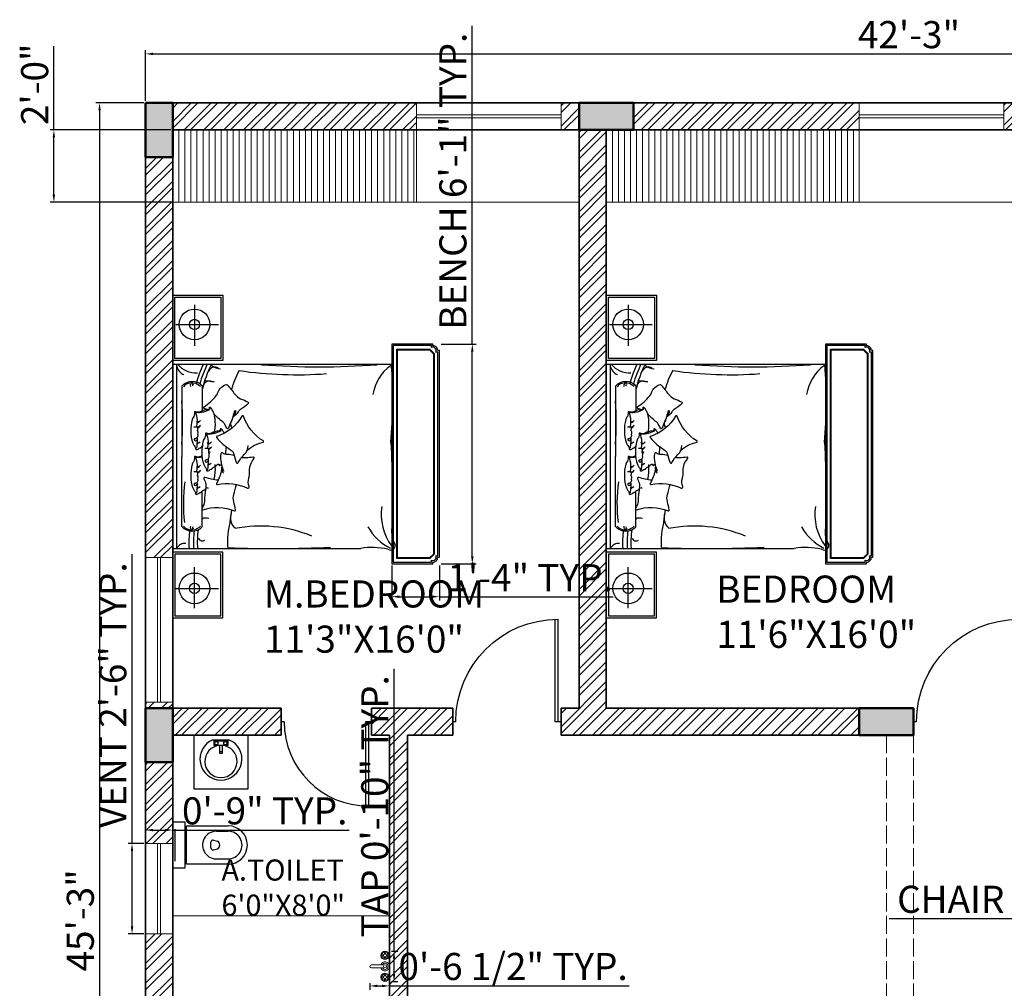
# Model space of a CAD drawing. Units: inches. Extents: x 4153 to 5577, y 785 to 1503.
# Tile 2 of 11: x 4153 to 4480, y 1150 to 1472. Entities that reach past the tile are written whole.
import ezdxf

# ---------------------------------------------------------------- set-up
doc = ezdxf.new("R2010")
doc.units = ezdxf.units.IN
doc.linetypes.add('ACAD_ISO02W100', pattern=[15, 12, -3])
for name, color, linetype, lineweight in [('A-ANNO-DIMS', 2, 'Continuous', 18), ('A-AREA-IDEN', 7, 'Continuous', 25), ('A-COLS', 7, 'Continuous', 50), ('A-DOOR', 3, 'Continuous', 25), ('A-FLOR-CASE', 32, 'Continuous', 18), ('A-FURN', 8, 'Continuous', 18), ('A-GLAZ', 4, 'Continuous', 18), ('A-WALL', 7, 'Continuous', 35), ('A-WALL-OVHD', 7, 'ACAD_ISO02W100', 18), ('Сантехника', 7, 'Continuous', 18)]:
    doc.layers.add(name, color=color, linetype=linetype, lineweight=lineweight)
doc.layers.add('A-FLOR-CASE-PATT', color=32, linetype='Continuous', lineweight=13, true_color=0xcd6928)
doc.layers.add('A-WALL-PATT', color=251, linetype='Continuous', lineweight=13, true_color=0x636466)
for name, color, linetype in [('FUR', 42, 'Continuous'), ('HA-FUR', 8, 'Continuous'), ('HA-P', 8, 'Continuous'), ('SAN', 5, 'Continuous'), ('SANTEH', 7, 'Continuous'), ('wood', 26, 'Continuous')]:
    doc.layers.add(name, color=color, linetype=linetype)
doc.styles.get("Standard").update_dxf_attribs({"font": 'arial.ttf'})
doc.dimstyles.new('ISO-25', dxfattribs={"dimtxt": 9, "dimasz": 2.5, "dimexe": 1.25, "dimexo": 0.625, "dimtad": 1, "dimlunit": 3, "dimtxsty": 'Standard', "dimcen": 2.5, "dimadec": 0, "dimazin": 0, "dimtfac": 1, "dimtmove": 0, "dimatfit": 3, "dimfxl": 1, "dimarcsym": 0})

# ---------------------------------------------------------------- blocks, each defined once
blk = doc.blocks.new('D1')
for p, q in [((1, 0), (1, 34)), ((2, 0), (2, 33.99)), ((0, 0), (2, 0)), ((35, 0), (36, 0))]:
    blk.add_line(p, q)
at = {"ltscale": 0.5}
blk.add_arc((1, 0), 34, 0, 90, dxfattribs=at)
blk = doc.blocks.new('D2')
for p, q in [((1, 0), (1, 28)), ((2, 0), (2, 27.98)), ((0, 0), (2, 0)), ((29, 0), (30, 0))]:
    blk.add_line(p, q)
at = {"ltscale": 0.5}
blk.add_arc((1, 0), 28, 0, 90, dxfattribs=at)
blk = doc.blocks.new('A$C0A42580C')
at = {"layer": 'SAN'}
for p, q in [((0.2873, 0.0301), (0.2873, 0.4484)), ((2.8678, 0.0301), (2.8678, 0.4484)), ((0.0949, 0.2135), (0.4958, 0.2135)), ((3.0601, 0.2135), (2.6592, 0.2135))]:
    blk.add_line(p, q, dxfattribs=at)
for centre, radius in [((0.2873, 0.2135), 0.15), ((2.8678, 0.2135), 0.15), ((0.2873, 0.2135), 0.05), ((2.8678, 0.2135), 0.05)]:
    blk.add_circle(centre, radius, dxfattribs=at)
at = {"layer": 'wood'}
for p, q in [((0.6775, 0.8851), (0.6775, 2.1392)), ((2.4775, 0.8016), (2.4775, 1.838)), ((2.4775, 0), (2.4775, 0.8016)), ((0.888, 0.289), (1.1327, 0.289)), ((1.5, 0.3423), (1.5016, 0.3142)), ((1.6633, 0.3438), (1.6434, 0.3761)), ((2.267, 0.289), (1.9163, 0.289)), ((1.2906, 0.2348), (1.2921, 0.2067)), ((1.4538, 0.2362), (1.434, 0.2685)), ((1.7287, 0.2348), (1.7302, 0.2067)), ((1.8919, 0.2362), (1.8721, 0.2685)), ((0.6775, 0.039), (2.4775, 0.039)), ((0.8909, 0.089), (1.5775, 0.089)), ((2.2642, 0.089), (1.5775, 0.089)), ((0.6775, 0), (2.4775, 0))]:
    blk.add_line(p, q, dxfattribs=at)
blk.add_lwpolyline([(0.6775, 0), (0.6775, 0.8851)], dxfattribs=at)
for points in [[(1.516, 0.7294, -0.128392), (1.4401, 0.8834, 0.70791), (1.427, 0.8863, -0.16964), (1.1848, 0.6919, 0.664036), (1.184, 0.6776, -0.184649), (1.3819, 0.4332, 0.662242), (1.3969, 0.4309, 0.078539), (1.5137, 0.5669, -0.1736), (1.5484, 0.5947, -0.02159), (1.6357, 0.6205, 0.697276), (1.6379, 0.6405, -0.093019), (1.5606, 0.699, 0.216632), (1.4719, 0.7371, -2.511293)], [(1.6795, 0.4818, 0.263265), (1.7191, 0.4839, -0.026108), (1.743, 0.4973, 0.027613), (1.7137, 0.4764, -0.089259), (1.8403, 0.429, 0.662242), (1.8528, 0.4376, -0.162037), (1.8882, 0.732, 0.676499), (1.8733, 0.748, -0.160513), (1.7901, 0.7439, 0.07473), (1.7202, 0.7523, -0.187721), (1.5966, 0.7963, 0.70791), (1.5851, 0.7895, -0.010003), (1.5921, 0.7143, -0.07079), (1.5891, 0.6719, 0.099539)], [(1.1211, 0.3454, 0.032543), (1.1095, 0.3091, -0.658965), (1.0917, 0.3063, 0.074753), (0.9887, 0.4234, 0.100988), (0.953, 0.4429, -0.270711), (0.8753, 0.5273, -0.276825), (0.8775, 0.5337, -0.014937), (0.9701, 0.6081, 0.134834), (1.0135, 0.6643, -0.023706), (1.0474, 0.7372, -0.664036), (1.0616, 0.7394, -0.035987), (1.119, 0.6627, 0.118631), (1.1415, 0.6412, -0.132738), (1.1955, 0.5864)], [(1.1759, 0.5928, 0.013884), (1.1549, 0.6131, 0.174178), (1.1437, 0.6177, 0.104076), (1.1358, 0.6165, 0.389829), (1.1324, 0.6097, 0.296089), (1.1415, 0.6019, -0.036701), (1.1572, 0.5985, -0.040547), (1.3022, 0.543, -0.70791), (1.3021, 0.5296, -0.016811), (1.2631, 0.5085, 0.11866), (1.2414, 0.4904, -0.048791), (1.1649, 0.4055, 0.103757)], [(1.5674, 0.601, 0.057807), (1.5606, 0.5339, -0.173425), (1.5457, 0.49, 0.589988), (1.5538, 0.4706, 0.137312), (1.7236, 0.4985, 0.137312)], [(1.8113, 0.4446, -0.069098), (1.7831, 0.3187, 0.658965), (1.7961, 0.3062, -0.049789), (1.8516, 0.3234, -0.103757), (1.8905, 0.3233, 0.055725), (2.0203, 0.3103, -0.11866), (2.0478, 0.304, 0.016811), (2.0881, 0.2856, 0.70791), (2.0989, 0.2936, -0.16964), (2.1104, 0.604, 0.664036), (2.1001, 0.6139, 0.023706), (2.0214, 0.597, -0.134834), (1.9505, 0.5976, 0.012748), (1.8522, 0.6228)], [(1.3107, 0.4764, 0.145733), (1.3069, 0.4677, 0.488583), (1.3089, 0.4657, -0.012138), (1.3131, 0.4661, -0.125673), (1.3213, 0.4646, -0.750706)], [(1.3153, 0.4751, -0.274893), (1.3379, 0.4529, 0.051436), (1.3468, 0.4293, -0.086628), (1.3532, 0.4078, 0.040196), (1.3593, 0.3772, -0.184744), (1.3556, 0.3344, -2.554464)], [(1.317, 0.4683, -0.060098), (1.3283, 0.4571, -0.16247), (1.3313, 0.4487, 0.120018), (1.3493, 0.3815, -0.060072), (1.3541, 0.3695, -0.13107), (1.3541, 0.3395, -0.024415), (1.3534, 0.3373, 0.070398), (1.3503, 0.3233, 0.528689), (1.3524, 0.3216, -0.069388), (1.3557, 0.3222, -0.158233), (1.4075, 0.3065, 0.085461), (1.4255, 0.2981, 0.147196), (1.6571, 0.3041, 0.10985), (1.6823, 0.3191, -0.179095), (1.7126, 0.3319, -2.318897)], [(1.1013, 0.3688, 0.145733), (1.0975, 0.3601, 0.488583), (1.0995, 0.3581, -0.012138), (1.1036, 0.3585, -0.125673), (1.1119, 0.357, -0.750706)], [(1.1059, 0.3675, -0.274893), (1.1285, 0.3453, 0.051436), (1.1373, 0.3217, -0.086628), (1.1438, 0.3003, 0.040196), (1.1499, 0.2696, -0.184744), (1.1462, 0.2269, -2.554464)], [(1.1076, 0.3607, -0.060098), (1.1189, 0.3495, -0.16247), (1.1219, 0.3411, 0.120018), (1.1399, 0.2739, -0.060072), (1.1447, 0.2619, -0.13107), (1.1447, 0.2319, -0.024415), (1.144, 0.2297, 0.070398), (1.1409, 0.2157, 0.528689), (1.143, 0.2141, -0.069388), (1.1463, 0.2146, -0.158233), (1.1981, 0.1989, 0.085461), (1.2161, 0.1905, 0.147196), (1.4477, 0.1965, 0.10985), (1.4728, 0.2115, -0.179095), (1.5032, 0.2244, -2.318897)], [(1.3509, 0.3219, -0.117141), (1.3688, 0.335, -0.025084), (1.4533, 0.348, 0.033691)], [(1.4359, 0.3803, -0.198519), (1.452, 0.3494, 0.826402), (1.4558, 0.349, 0.095956), (1.4561, 0.3528, 0.242899), (1.4461, 0.3686, -17.523452)], [(1.5447, 0.3525, -0.083557), (1.507, 0.3546, 0.203162), (1.4851, 0.3792, -0.208037), (1.5043, 0.3409, 0.124669), (1.4432, 0.3469, 0.965934)], [(1.5394, 0.3688, 0.145733), (1.5356, 0.3601, 0.488583), (1.5376, 0.3581, -0.012138), (1.5418, 0.3585, -0.125673), (1.55, 0.357, -0.750706)], [(1.5447, 0.3525, -0.008229), (1.5728, 0.3519, 0.033691)], [(1.5728, 0.3519, -0.46905), (1.6152, 0.321, 0.420988), (1.62, 0.3169, 0.857652), (1.6221, 0.3484, 0.548526)], [(1.603, 0.3451, -0.099719), (1.6221, 0.3484, 0.102691)], [(1.6214, 0.3487, -0.010168), (1.6558, 0.3447, 0.033691), (1.6907, 0.3423, -0.220869), (1.7148, 0.3311, -0.288972)], [(1.1415, 0.2143, -0.117141), (1.1594, 0.2274, -0.025084), (1.2439, 0.2405, 0.033691)], [(1.2265, 0.2728, -0.198519), (1.2426, 0.2418, 0.826402), (1.2463, 0.2415, 0.095956), (1.2467, 0.2452, 0.242899), (1.2366, 0.2611, -17.523452)], [(1.3353, 0.2449, -0.083557), (1.2976, 0.247, 0.203162), (1.2757, 0.2717, -0.208037), (1.2948, 0.2333, 0.124669), (1.2338, 0.2393, 0.965934)], [(1.3353, 0.2449, -0.008229), (1.3633, 0.2443, 0.033691)], [(1.3633, 0.2443, -0.46905), (1.4058, 0.2134, 0.420988), (1.4106, 0.2093, 0.857652), (1.4127, 0.2408, 0.548526)], [(1.3936, 0.2375, -0.099719), (1.4127, 0.2408, 0.102691)], [(1.412, 0.2411, -0.010168), (1.4464, 0.2371, 0.033691), (1.4812, 0.2348, -0.220869), (1.5054, 0.2235, -0.288972)], [(1.5721, 0.286, 0.022869), (1.578, 0.2739, -0.060072), (1.5828, 0.2619, -0.13107), (1.5828, 0.2319, -0.024415), (1.5821, 0.2297, 0.070398), (1.579, 0.2157, 0.528689), (1.5811, 0.2141, -0.069388), (1.5844, 0.2146, -0.158233), (1.6362, 0.1989, 0.085461), (1.6542, 0.1905, 0.147196), (1.8858, 0.1965, 0.10985), (1.911, 0.2115, -0.179095), (1.9413, 0.2244, -2.318897)], [(1.5796, 0.2143, -0.117141), (1.5975, 0.2274, -0.025084), (1.682, 0.2405, 0.033691)], [(1.5838, 0.2873, 0.023398), (1.588, 0.2696, -0.184744), (1.5843, 0.2269, -2.554464)], [(1.6646, 0.2728, -0.198519), (1.6807, 0.2418, 0.826402), (1.6845, 0.2415, 0.095956), (1.6848, 0.2452, 0.242899), (1.6748, 0.2611, -17.523452)], [(1.7734, 0.2449, -0.083557), (1.7357, 0.247, 0.203162), (1.7138, 0.2717, -0.208037), (1.733, 0.2333, 0.124669), (1.6719, 0.2393, 0.965934)], [(1.7734, 0.2449, -0.008229), (1.8015, 0.2443, 0.033691)], [(1.8015, 0.2443, -0.46905), (1.8439, 0.2134, 0.420988), (1.8487, 0.2093, 0.857652), (1.8508, 0.2408, 0.548526)], [(1.8317, 0.2375, -0.099719), (1.8508, 0.2408, 0.102691)], [(1.8501, 0.2411, -0.010168), (1.8845, 0.2371, 0.033691), (1.9193, 0.2348, -0.220869), (1.9435, 0.2235, -0.288972)]]:
    blk.add_lwpolyline(points, format="xyb", dxfattribs=at)
for points in [[(0.64, 0), (0, 0), (0, 0.49), (0.64, 0.49)], [(2.515, 0), (3.155, 0), (3.155, 0.49), (2.515, 0.49)], [(0.62, 0.02), (0.02, 0.02), (0.02, 0.47), (0.62, 0.47)], [(2.535, 0.02), (3.135, 0.02), (3.135, 0.47), (2.535, 0.47)]]:
    blk.add_lwpolyline(points, close=True, dxfattribs=at)
for centre, radius, start, end in [((1.0344, -2.14), 4.292, 84.56078, 94.7164), ((1.0494, 2.4026), 0.4515, 217.47941, 260.35986), ((2.0208, -11.0786), 13.2288, 88.75549, 92.51133), ((2.1491, 2.5471), 0.5083, 260.65485, 306.44155), ((2.3125, 2.3833), 0.2443, 254.1515, 300.95574), ((2.0168, 2.3573), 0.5127, 299.08175, 333.44367), ((2.4501, 2.1309), 0.0445, 324.18954, 118.92203), ((3.1371, 1.9502), 0.669, 166.6404, 189.65708), ((-7.0839, 1.4328), 7.7858, 355.84817, 4.15183), ((-7.2439, 0.9937), 9.7233, 357.34474, 3.23068), ((-3.167, 1.2143), 3.9465, 351.77286, 4.18386), ((3.5803, 0.8622), 1.3213, 157.81295, 191.15154), ((1.1611, 1.4181), 0.8768, 241.21362, 254.41879), ((1.7861, -2.1601), 2.7557, 80.89877, 83.46656), ((2.181, 0.6859), 0.1221, 247.37754, 321.13165), ((1.2583, 0.6364), 0.0695, 238.58923, 301.92671), ((1.3546, 0.4469), 0.0529, 114.21284, 146.15395), ((2.6126, -2.3504), 3.1201, 113.83178, 114.21284), ((1.4714, 0.0722), 0.4528, 80.62397, 88.74059), ((1.4035, -0.3388), 0.8693, 79.71489, 80.62397), ((1.6301, 0.4539), 0.0342, 31.14095, 54.95422), ((2.4192, 1.3819), 0.8461, 255.77539, 273.25587), ((0.5904, 0.4689), 0.13, 317.38218, 359.70393), ((0.7723, 0.4131), 0.0674, 147.68233, 245.79865), ((0.0312, 0.4583), 0.8174, 350.42368, 356.2506), ((1.1452, 0.3394), 0.0529, 114.21284, 146.15395), ((2.4032, -2.458), 3.1201, 113.55686, 114.21284), ((1.2046, 0.2912), 0.121, 99.42032, 113.55686), ((1.2774, -0.1478), 0.5659, 95.90379, 99.42032), ((1.2626, -0.005), 0.4223, 88.74059, 95.90379), ((1.2619, -0.0354), 0.4528, 80.62397, 88.74059), ((1.1941, -0.4464), 0.8693, 79.45871, 80.62397), ((1.6709, 0.4489), 0.0156, 131.9623, 212.08127), ((1.6729, 0.4422), 0.0178, 140.41793, 157.63267), ((1.7007, -0.005), 0.4223, 88.74059, 95.90379), ((1.7235, 0.4818), 0.0777, 212.08127, 227.364), ((1.6635, 0.4499), 0.00568, 95.52245, 140.41793), ((1.5664, 0.4154), 0.1086, 24.20989, 31.14095), ((1.6627, 0.4587), 0.00309, 275.52245, 24.20989), ((1.6391, 0.3902), 0.0469, 17.32618, 47.364), ((1.7106, 0.4125), 0.028, 197.32618, 226.17302), ((1.6431, 0.3422), 0.0695, 26.61764, 46.17302), ((1.7001, -0.0354), 0.4528, 80.62397, 88.74059), ((1.6322, -0.4464), 0.8693, 78.43923, 80.62397), ((1.1611, 1.3191), 1.0568, 242.76671, 257.10398), ((1.1611, 1.3191), 1.0937, 243.75553, 254.4906), ((1.1611, 1.2816), 1.0937, 243.75553, 254.38927), ((0.9021, 0.3562), 0.0605, 155.8342, 254.41058), ((0.9846, 0.1903), 0.1381, 134.39284, 227.23745), ((1.4207, 0.3463), 0.0342, 31.14095, 54.95422), ((1.4614, 0.3413), 0.0156, 131.9623, 212.08127), ((1.4635, 0.3347), 0.0178, 140.41793, 157.63267), ((1.4541, 0.3424), 0.00568, 95.52245, 140.41793), ((1.357, 0.3078), 0.1086, 24.20989, 31.14095), ((1.4533, 0.3511), 0.00309, 275.52245, 24.20989), ((1.5012, 0.305), 0.028, 197.32618, 226.17302), ((1.8202, 0.431), 0.1287, 206.61764, 215.96192), ((1.715, 0.3349), 0.00379, 207.1817, 328.02977), ((1.6975, 0.3419), 0.023, 350.76434, 35.96192), ((1.7058, 0.3406), 0.0145, 328.02977, 350.76434), ((1.9016, 0.3347), 0.0178, 140.41793, 157.63267), ((1.9522, 0.3743), 0.0777, 212.08127, 227.364), ((1.8922, 0.3424), 0.00568, 95.52245, 140.41793), ((1.8678, 0.2827), 0.0469, 17.32618, 47.364), ((1.9393, 0.305), 0.028, 197.32618, 226.17302), ((2.2511, 0.3256), 0.071, 155.86842, 211.04513), ((2.1704, 0.1903), 0.1381, 312.76255, 45.60716), ((2.3616, 0.2915), 0.0419, 290.78583, 35.36309), ((0.5293, 0.2241), 0.2307, 309.63048, 4.27465), ((0.8396, 0.185), 0.0112, 314.89662, 45.10338), ((0.8413, 0.1846), 0.0128, 299.47062, 57.44416), ((0.8802, 0.1371), 0.0592, 81.47786, 123.11925), ((0.8698, 0.1793), 0.0229, 77.14902, 159.1786), ((0.9986, 0.1735), 0.1427, 136.58239, 164.9725), ((1.4337, 0.2347), 0.0695, 26.61764, 46.17302), ((1.6108, 0.3235), 0.1287, 206.61764, 215.96192), ((1.5055, 0.2273), 0.00379, 207.1817, 328.02977), ((1.4881, 0.2344), 0.023, 350.76434, 35.96192), ((1.4964, 0.233), 0.0145, 328.02977, 350.76434), ((1.8718, 0.2347), 0.0695, 26.61764, 46.17302), ((2.0489, 0.3235), 0.1287, 206.61764, 215.96192), ((1.9436, 0.2273), 0.00379, 207.1817, 328.02977), ((1.9262, 0.2344), 0.023, 350.76434, 35.96192), ((1.9345, 0.233), 0.0145, 328.02977, 350.76434), ((2.1565, 0.1735), 0.1427, 15.0275, 43.41761), ((2.2749, 0.1371), 0.0592, 56.88075, 98.52214), ((2.2853, 0.1793), 0.0229, 20.8214, 102.85098), ((2.4192, 1.2667), 1.0261, 263.09035, 273.25587), ((2.3138, 0.1846), 0.0128, 122.55584, 240.52938), ((2.3154, 0.185), 0.0112, 134.89662, 225.10338), ((2.4192, 1.2667), 1.0629, 263.94374, 273.25587), ((0.6729, 0.151), 0.1135, 279.23824, 338.73819), ((0.8844, 0.2286), 0.0569, 229.70587, 281.11527), ((0.9466, 0.1765), 0.0862, 185.53723, 234.68694), ((1.2481, -2.5919), 2.6893, 85.4722, 94.5278), ((2.0447, 1.7022), 1.5979, 262.13639, 276.48786), ((2.2085, 0.1765), 0.0862, 305.31306, 354.46277), ((2.2706, 0.2286), 0.0569, 258.88473, 310.29413), ((2.4192, 1.2218), 1.0629, 263.23622, 273.25587), ((2.508, 0.1152), 0.0792, 169.94668, 248.24015)]:
    blk.add_arc(centre, radius, start, end, dxfattribs=at)
blk = doc.blocks.new('A$C623F1DA0')
at = {"layer": 'FUR'}
blk.add_lwpolyline([(0.628, 2.912, 0.414214), (0.562, 2.978), (0.562, 3), (0, 3), (0, 0), (0.562, 0), (0.562, 0.022, 0.414214), (0.628, 0.088), (0.65, 0.088), (0.65, 2.912)], format="xyb", close=True, dxfattribs=at)
at = {"layer": 'HA-FUR'}
blk.add_lwpolyline([(0.603, 2.892, 0.710288), (0.542, 2.953), (0.542, 2.98), (0.02, 2.98), (0.02, 0.02), (0.542, 0.02), (0.542, 0.047, 0.710288), (0.603, 0.108), (0.63, 0.108), (0.63, 2.892)], format="xyb", close=True, dxfattribs=at)
at = {"layer": 'HA-P'}
for points in [[(0.07, 2.93), (0.521, 2.93), (0.58, 2.871), (0.58, 0.129), (0.521, 0.07), (0.07, 0.07)], [(0.08, 2.92), (0.517, 2.92), (0.57, 2.867), (0.57, 0.133), (0.517, 0.08), (0.08, 0.08)]]:
    blk.add_lwpolyline(points, close=True, dxfattribs=at)
blk = doc.blocks.new('Faucet - Bathroom top')
for p, q in [((-4.107, 0.125), (-4.375, 0.125)), ((-3.75, 0.4788), (-3.75, 0.75)), ((-3.5, 0.482), (-3.5, 0.75)), ((-3.1461, 0.125), (-2.875, 0.125)), ((3.143, 0.125), (2.875, 0.125)), ((3.5, 0.4788), (3.5, 0.75)), ((3.75, 0.482), (3.75, 0.75)), ((4.1039, 0.125), (4.375, 0.125)), ((-4.1039, -0.125), (-4.375, -0.125)), ((-3.75, -0.4821), (-3.75, -0.75)), ((-3.5, -0.4789), (-3.5, -0.75)), ((-3.143, -0.125), (-2.875, -0.125)), ((-0.5, -0.8639), (-0.5, -4.5)), ((0.5, -4.5), (0.5, -0.8631)), ((3.1461, -0.125), (2.875, -0.125)), ((3.5, -0.4821), (3.5, -0.75)), ((3.75, -0.4789), (3.75, -0.75)), ((4.107, -0.125), (4.375, -0.125))]:
    blk.add_line(p, q)
for centre, radius in [((-3.625, 0), 1.375), ((-4.625, 0), 0.2795), ((-3.625, 0), 0.5), ((-3.625, 1), 0.2795), ((-2.625, 0), 0.2795), ((0, 0), 0.5), ((3.625, 0), 1.375), ((2.625, 0), 0.2795), ((3.625, 0), 0.5), ((3.625, 1), 0.2795), ((4.625, 0), 0.2795), ((-3.625, -1), 0.2795), ((3.625, -1), 0.2795)]:
    blk.add_circle(centre, radius)
for centre, radius, start, end in [((-3.625, 0), 1, 105.2407, 164.2093), ((-3.625, 0), 1, 16.44125, 74.07887), ((0, 0), 1.5, 289.6514, 250.3603), ((0, 0), 1, 300.3431, 239.7554), ((3.625, 0), 1, 106.12, 164.0884), ((3.625, 0), 1, 16.23422, 73.90469), ((-3.625, 0), 1, 196.2342, 253.9047), ((-3.625, 0), 1, 286.12, 344.0884), ((3.625, 0), 1, 196.4413, 254.0789), ((3.625, 0), 1, 285.2407, 344.2093), ((0, -4.5), 0.5, 180, 0)]:
    blk.add_arc(centre, radius, start, end)
blk = doc.blocks.new('y3')
at = {"layer": 'SANTEH', "ltscale": 5}
for p, q in [((37.5, 130.7), (37.5, 520.7)), ((87.5, 410.7), (87.5, 520.7)), ((346.6, 426.1), (347.5, 520.7)), ((397.5, 520.7), (397.5, 130.7)), ((171.9, 384.5), (181.1, 421.3)), ((263.1, 384.5), (253.9, 421.3)), ((244.3, 357.8), (190.7, 357.8)), ((397.5, 130.7), (37.5, 130.7)), ((67.5, 20.7), (367.5, 20.7))]:
    blk.add_line(p, q, dxfattribs=at)
blk.add_lwpolyline([(0, 115), (435, 115), (435, 0), (0, 0), (0, 115)], dxfattribs=at)
for centre, radius, start, end in [((217.5, 520.7), 180, 0, 180), ((217.5, 520.7), 130, 359.15795, 180), ((217.5, 410.7), 130, 180, 5.98548), ((190.7, 377.8), 20, 160.50385, 270), ((217.5, 399.9), 42.2, 30.52342, 149.47658), ((244.3, 377.8), 20, 270, 19.49615)]:
    blk.add_arc(centre, radius, start, end, dxfattribs=at)
blk = doc.blocks.new('r11')
at = {"layer": 'SANTEH', "ltscale": 5}
for p, q in [((0, 0), (600, 0)), ((0, -600), (0, 0)), ((600, 0), (600, -600)), ((210, -50), (390, -50)), ((210, -50), (210, -50)), ((224, -63), (376, -63)), ((224, -113), (224, -63)), ((233, -79), (249, -69)), ((233, -98), (233, -79)), ((249, -107), (233, -98)), ((249, -69), (266, -79)), ((266, -98), (249, -107)), ((266, -79), (266, -98)), ((334, -79), (351, -69)), ((334, -98), (334, -79)), ((351, -107), (334, -98)), ((351, -69), (367, -79)), ((367, -98), (351, -107)), ((367, -79), (367, -98)), ((376, -63), (376, -113)), ((376, -113), (224, -113)), ((288, -202), (288, -113)), ((312, -184), (288, -184)), ((312, -202), (288, -202)), ((312, -113), (312, -202)), ((600, -600), (0, -600))]:
    blk.add_line(p, q, dxfattribs=at)
for centre, radius, start, end in [((300, -266), 234, 112.5, 67.5), ((300, -293), 180, 93.8183, 86.1817)]:
    blk.add_arc(centre, radius, start, end, dxfattribs=at)
blk = doc.blocks.new('*D21')
at = {"layer": 'A-ANNO-DIMS', "color": 0, "lineweight": -2, "transparency": 16777216}
for p, q in [((4194.93, 1445.11), (4194.93, 1461.99)), ((4701.93, 1445.11), (4701.93, 1461.99)), ((4197.43, 1460.74), (4699.43, 1460.74))]:
    blk.add_line(p, q, dxfattribs=at)
at = {"layer": 'A-ANNO-DIMS', "color": 0, "transparency": 16777216}
for points in [[(4197.43, 1461.16), (4197.43, 1460.33), (4194.93, 1460.74)], [(4699.43, 1461.16), (4699.43, 1460.33), (4701.93, 1460.74)]]:
    blk.add_solid(points, dxfattribs=at)
at = {"layer": 'Defpoints', "color": 0, "transparency": 16777216}
for p in [(4701.93, 1460.74), (4194.93, 1444.49), (4701.93, 1444.49)]:
    blk.add_point(p, dxfattribs=at)
at = {"layer": 'A-ANNO-DIMS', "color": 0, "transparency": 16777216, "insert": (4448.43, 1465.97), "char_height": 9, "attachment_point": 5}
blk.add_mtext('42\'-3"', dxfattribs=at)
blk = doc.blocks.new('*D22')
at = {"layer": 'A-ANNO-DIMS', "color": 0, "lineweight": -2, "transparency": 16777216}
for p, q in [((4194.3, 1444.49), (4178.39, 1444.49)), ((4179.64, 1441.99), (4179.64, 903.99)), ((4194.3, 901.49), (4178.39, 901.49))]:
    blk.add_line(p, q, dxfattribs=at)
at = {"layer": 'A-ANNO-DIMS', "color": 0, "transparency": 16777216}
for points in [[(4179.23, 1441.99), (4180.06, 1441.99), (4179.64, 1444.49)], [(4179.23, 903.99), (4180.06, 903.99), (4179.64, 901.49)]]:
    blk.add_solid(points, dxfattribs=at)
at = {"layer": 'Defpoints', "color": 0, "transparency": 16777216}
for p in [(4194.93, 1444.49), (4179.64, 901.49), (4194.93, 901.49)]:
    blk.add_point(p, dxfattribs=at)
at = {"layer": 'A-ANNO-DIMS', "color": 0, "transparency": 16777216, "insert": (4174.42, 1172.99), "char_height": 9, "attachment_point": 5, "rotation": 90}
blk.add_mtext('45\'-3"', dxfattribs=at)
blk = doc.blocks.new('WINDOW-48IN')
for p, q in [((0, 9), (0, 0)), ((48, 9), (48, 0)), ((0, 5), (48, 5)), ((0, 4), (48, 4))]:
    blk.add_line(p, q)
blk = doc.blocks.new('VENT-WINDOW-30IN')
for p, q in [((9, 30), (0, 30)), ((4, 0), (4, 30)), ((5, 0), (5, 30)), ((9, 0), (0, 0))]:
    blk.add_line(p, q)
blk = doc.blocks.new('COL-9X18IN')
at = {"transparency": 33554687}
h = blk.add_hatch(color=256, dxfattribs=at)
h.dxf.hatch_style = 1
h.paths.add_polyline_path([(9, 18), (0, 18), (0, 0), (9, 0)])
blk.add_lwpolyline([(0, 18), (9, 18), (9, 0), (0, 0)], close=True)
blk = doc.blocks.new('*D110')
at = {"layer": 'A-ANNO-DIMS', "color": 0, "lineweight": -2, "transparency": 16777216}
for p, q in [((4190.43, 1198.49), (4190.43, 1294.59)), ((4194.3, 1198.49), (4189.18, 1198.49)), ((4190.43, 1170.99), (4190.43, 1195.99)), ((4194.3, 1168.49), (4189.18, 1168.49))]:
    blk.add_line(p, q, dxfattribs=at)
at = {"layer": 'A-ANNO-DIMS', "color": 0, "transparency": 16777216}
for points in [[(4190.01, 1195.99), (4190.84, 1195.99), (4190.43, 1198.49)], [(4190.01, 1170.99), (4190.84, 1170.99), (4190.43, 1168.49)]]:
    blk.add_solid(points, dxfattribs=at)
at = {"layer": 'Defpoints', "color": 0, "transparency": 16777216}
for p in [(4190.43, 1198.49), (4194.93, 1198.49), (4194.93, 1168.49)]:
    blk.add_point(p, dxfattribs=at)
at = {"layer": 'A-ANNO-DIMS', "color": 0, "transparency": 16777216, "insert": (4185.21, 1247.79), "char_height": 9, "attachment_point": 5, "rotation": 90}
blk.add_mtext('VENT 2\'-6" TYP.', dxfattribs=at)
blk = doc.blocks.new('*D111')
at = {"layer": 'A-ANNO-DIMS', "color": 0, "lineweight": -2, "transparency": 16777216}
for p, q in [((4194.93, 1199.11), (4194.93, 1204.24)), ((4203.93, 1199.11), (4203.93, 1204.24)), ((4197.43, 1202.99), (4201.43, 1202.99)), ((4203.93, 1202.99), (4262.54, 1202.99))]:
    blk.add_line(p, q, dxfattribs=at)
at = {"layer": 'A-ANNO-DIMS', "color": 0, "transparency": 16777216}
for points in [[(4197.43, 1203.41), (4197.43, 1202.57), (4194.93, 1202.99)], [(4201.43, 1203.41), (4201.43, 1202.57), (4203.93, 1202.99)]]:
    blk.add_solid(points, dxfattribs=at)
at = {"layer": 'Defpoints', "color": 0, "transparency": 16777216}
for p in [(4203.93, 1202.99), (4194.93, 1198.49), (4203.93, 1198.49)]:
    blk.add_point(p, dxfattribs=at)
at = {"layer": 'A-ANNO-DIMS', "color": 0, "transparency": 16777216, "insert": (4234.48, 1208.21), "char_height": 9, "attachment_point": 5}
blk.add_mtext('0\'-9" TYP.', dxfattribs=at)
blk = doc.blocks.new('*D114')
at = {"layer": 'A-ANNO-DIMS', "color": 0, "lineweight": -2, "transparency": 16777216}
for p, q in [((4303.43, 1364.36), (4303.43, 1470.08)), ((4293.11, 1364.36), (4304.68, 1364.36)), ((4303.43, 1293.93), (4303.43, 1361.86)), ((4293.11, 1291.43), (4304.68, 1291.43))]:
    blk.add_line(p, q, dxfattribs=at)
at = {"layer": 'A-ANNO-DIMS', "color": 0, "transparency": 16777216}
for points in [[(4303.01, 1361.86), (4303.84, 1361.86), (4303.43, 1364.36)], [(4303.01, 1293.93), (4303.84, 1293.93), (4303.43, 1291.43)]]:
    blk.add_solid(points, dxfattribs=at)
at = {"layer": 'Defpoints', "color": 0, "transparency": 16777216}
for p in [(4292.49, 1364.36), (4303.43, 1364.36), (4292.49, 1291.43)]:
    blk.add_point(p, dxfattribs=at)
at = {"layer": 'A-ANNO-DIMS', "color": 0, "transparency": 16777216, "insert": (4298.15, 1418.47), "char_height": 9, "attachment_point": 5, "rotation": 90}
blk.add_mtext('BENCH 6\'-1" TYP.', dxfattribs=at)
blk = doc.blocks.new('*D115')
at = {"layer": 'A-ANNO-DIMS', "color": 0, "lineweight": -2, "transparency": 16777216}
for p, q in [((4276.69, 1290.81), (4276.69, 1279.24)), ((4292.49, 1290.81), (4292.49, 1279.24)), ((4279.19, 1280.49), (4289.99, 1280.49)), ((4292.49, 1280.49), (4350.25, 1280.49))]:
    blk.add_line(p, q, dxfattribs=at)
at = {"layer": 'A-ANNO-DIMS', "color": 0, "transparency": 16777216}
for points in [[(4279.19, 1280.91), (4279.19, 1280.08), (4276.69, 1280.49)], [(4289.99, 1280.91), (4289.99, 1280.08), (4292.49, 1280.49)]]:
    blk.add_solid(points, dxfattribs=at)
at = {"layer": 'Defpoints', "color": 0, "transparency": 16777216}
for p in [(4276.69, 1291.43), (4292.49, 1291.43), (4292.49, 1280.49)]:
    blk.add_point(p, dxfattribs=at)
at = {"layer": 'A-ANNO-DIMS', "color": 0, "transparency": 16777216, "insert": (4322.62, 1285.64), "char_height": 9, "attachment_point": 5}
blk.add_mtext('1\'-4" TYP.', dxfattribs=at)
blk = doc.blocks.new('*D116')
at = {"layer": 'A-ANNO-DIMS', "color": 0, "lineweight": -2, "transparency": 16777216}
for p, q in [((4277.43, 1162.74), (4277.43, 1256.51)), ((4276.55, 1162.74), (4278.68, 1162.74)), ((4277.43, 1155.24), (4277.43, 1160.24)), ((4276.55, 1152.74), (4278.68, 1152.74))]:
    blk.add_line(p, q, dxfattribs=at)
at = {"layer": 'A-ANNO-DIMS', "color": 0, "transparency": 16777216}
for points in [[(4277.01, 1160.24), (4277.84, 1160.24), (4277.43, 1162.74)], [(4277.01, 1155.24), (4277.84, 1155.24), (4277.43, 1152.74)]]:
    blk.add_solid(points, dxfattribs=at)
at = {"layer": 'Defpoints', "color": 0, "transparency": 16777216}
for p in [(4275.93, 1162.74), (4277.43, 1162.74), (4275.93, 1152.74)]:
    blk.add_point(p, dxfattribs=at)
at = {"layer": 'A-ANNO-DIMS', "color": 0, "transparency": 16777216, "insert": (4272.21, 1210.88), "char_height": 9, "attachment_point": 5, "rotation": 90}
blk.add_mtext('TAP 0\'-10" TYP.', dxfattribs=at)
blk = doc.blocks.new('*D117')
at = {"layer": 'A-ANNO-DIMS', "color": 0, "lineweight": -2, "transparency": 16777216}
for p, q in [((4269.43, 1152.11), (4269.43, 1149.99)), ((4271.93, 1151.24), (4273.43, 1151.24)), ((4275.93, 1152.11), (4275.93, 1149.99)), ((4275.93, 1151.24), (4355.51, 1151.24))]:
    blk.add_line(p, q, dxfattribs=at)
at = {"layer": 'A-ANNO-DIMS', "color": 0, "transparency": 16777216}
for points in [[(4271.93, 1151.66), (4271.93, 1150.82), (4269.43, 1151.24)], [(4273.43, 1151.66), (4273.43, 1150.82), (4275.93, 1151.24)]]:
    blk.add_solid(points, dxfattribs=at)
at = {"layer": 'Defpoints', "color": 0, "transparency": 16777216}
for p in [(4269.43, 1152.74), (4275.93, 1152.74), (4275.93, 1151.24)]:
    blk.add_point(p, dxfattribs=at)
at = {"layer": 'A-ANNO-DIMS', "color": 0, "transparency": 16777216, "insert": (4316.97, 1156.52), "char_height": 9, "attachment_point": 5}
blk.add_mtext('0\'-6 1/2" TYP.', dxfattribs=at)
blk = doc.blocks.new('*D128')
at = {"layer": 'A-ANNO-DIMS', "color": 0, "lineweight": -2, "transparency": 16777216}
for p, q in [((4542.96, 1178.31), (4542.96, 1172.3)), ((4578.86, 1178.31), (4578.86, 1172.3)), ((4542.96, 1173.55), (4441.84, 1173.55)), ((4576.36, 1173.55), (4545.46, 1173.55))]:
    blk.add_line(p, q, dxfattribs=at)
at = {"layer": 'A-ANNO-DIMS', "color": 0, "transparency": 16777216}
for points in [[(4545.46, 1173.96), (4545.46, 1173.13), (4542.96, 1173.55)], [(4576.36, 1173.96), (4576.36, 1173.13), (4578.86, 1173.55)]]:
    blk.add_solid(points, dxfattribs=at)
at = {"layer": 'Defpoints', "color": 0, "transparency": 16777216}
for p in [(4542.96, 1178.93), (4578.86, 1178.93), (4542.96, 1173.55)]:
    blk.add_point(p, dxfattribs=at)
at = {"layer": 'A-ANNO-DIMS', "color": 0, "transparency": 16777216, "insert": (4491.15, 1178.83), "char_height": 9, "attachment_point": 5}
blk.add_mtext('CHAIR 3\'-0" TYP.', dxfattribs=at)
blk = doc.blocks.new('*D161')
at = {"layer": 'A-ANNO-DIMS', "color": 0, "lineweight": -2, "transparency": 16777216}
for p, q in [((4164.48, 1435.49), (4164.48, 1463.32)), ((4203.3, 1435.49), (4163.23, 1435.49)), ((4164.48, 1413.99), (4164.48, 1432.99)), ((4203.3, 1411.49), (4163.23, 1411.49))]:
    blk.add_line(p, q, dxfattribs=at)
at = {"layer": 'A-ANNO-DIMS', "color": 0, "transparency": 16777216}
for points in [[(4164.06, 1432.99), (4164.89, 1432.99), (4164.48, 1435.49)], [(4164.06, 1413.99), (4164.89, 1413.99), (4164.48, 1411.49)]]:
    blk.add_solid(points, dxfattribs=at)
at = {"layer": 'Defpoints', "color": 0, "transparency": 16777216}
for p in [(4164.48, 1435.49), (4203.93, 1435.49), (4203.93, 1411.49)]:
    blk.add_point(p, dxfattribs=at)
at = {"layer": 'A-ANNO-DIMS', "color": 0, "transparency": 16777216, "insert": (4159.26, 1450.65), "char_height": 9, "attachment_point": 5, "rotation": 90}
blk.add_mtext('2\'-0"', dxfattribs=at)

msp = doc.modelspace()

# ---------------------------------------------------------------- hatches: boundary and pattern name
at = {"layer": 'A-FLOR-CASE-PATT'}
h = msp.add_hatch(dxfattribs=at)
h.set_pattern_fill('ANSI31', color=256, scale=0.629921, angle=45, style=0)
h.paths.add_polyline_path([(4203.927, 1411.488), (4284.927, 1411.488), (4284.927, 1435.488), (4203.927, 1435.488)])
h = msp.add_hatch(dxfattribs=at)
h.set_pattern_fill('ANSI31', color=256, scale=0.629921, angle=45, style=0)
h.paths.add_polyline_path([(4347.927, 1411.488), (4431.927, 1411.488), (4431.927, 1435.488), (4347.927, 1435.488)])
at = {"layer": 'A-WALL-PATT', "transparency": 33554687}
h = msp.add_hatch(dxfattribs=at)
h.set_pattern_fill('ANSI32', color=256, scale=0.49)
h.paths.add_polyline_path([(4344.927, 1138.488), (4281.927, 1138.488), (4281.927, 1234.488), (4296.927, 1234.488), (4296.927, 1243.488), (4269.927, 1243.488), (4269.927, 1234.488), (4275.927, 1234.488), (4275.927, 1138.488), (4203.927, 1138.488), (4203.927, 1168.488), (4194.927, 1168.488), (4194.927, 1088.988), (4203.927, 1088.988), (4203.927, 1129.488), (4338.927, 1129.488), (4338.927, 1105.488), (4344.927, 1105.488)])
h.paths.add_polyline_path([(4203.927, 1040.988), (4194.927, 1040.988), (4194.927, 1009.488), (4203.927, 1009.488)])
h.paths.add_polyline_path([(4278.927, 1000.488), (4203.927, 1000.488), (4203.927, 991.488), (4278.927, 991.488)])
h.paths.add_polyline_path([(4203.927, 991.488), (4194.927, 991.488), (4194.927, 910.488), (4203.927, 910.488)])
h.paths.add_polyline_path([(4335.927, 907.488), (4203.927, 907.488), (4203.927, 901.488), (4335.927, 901.488)])
h.paths.add_polyline_path([(4344.927, 1057.488), (4338.927, 1057.488), (4338.927, 1000.488), (4344.927, 1000.488)])
h.paths.add_polyline_path([(4335.927, 1000.488), (4326.927, 1000.488), (4326.927, 991.488), (4335.927, 991.488)])
h.paths.add_polyline_path([(4368.927, 1000.488), (4344.927, 1000.488), (4344.927, 991.488), (4368.927, 991.488)])
h.paths.add_polyline_path([(4440.927, 1000.488), (4416.927, 1000.488), (4416.927, 991.488), (4440.927, 991.488)])
h.paths.add_polyline_path([(4449.927, 1120.488), (4440.927, 1120.488), (4440.927, 1000.488), (4449.927, 1000.488)])
h.paths.add_polyline_path([(4473.927, 1000.488), (4458.927, 1000.488), (4458.927, 991.488), (4473.927, 991.488)])
h.paths.add_polyline_path([(4638.927, 1000.488), (4545.927, 1000.488), (4545.927, 991.488), (4638.927, 991.488)])
h.paths.add_polyline_path([(4701.927, 1036.488), (4692.927, 1036.488), (4692.927, 1009.488), (4701.927, 1009.488)])
h.paths.add_polyline_path([(4692.927, 1000.488), (4686.927, 1000.488), (4686.927, 991.488), (4692.927, 991.488)])
h.paths.add_polyline_path([(4701.927, 1132.488), (4692.927, 1132.488), (4692.927, 1108.488), (4701.927, 1108.488)])
h.paths.add_polyline_path([(4701.927, 1225.488), (4692.927, 1225.488), (4692.927, 1204.488), (4701.927, 1204.488)])
h.paths.add_polyline_path([(4650.927, 1243.488), (4560.927, 1243.488), (4560.927, 1265.228), (4560.927, 1381.488), (4650.927, 1381.488), (4650.927, 1393.488), (4644.927, 1393.488), (4644.927, 1387.488), (4560.927, 1387.488), (4560.927, 1435.488), (4551.927, 1435.488), (4551.927, 1354.488), (4530.927, 1354.488), (4530.927, 1348.488), (4551.927, 1348.488), (4551.927, 1309.488), (4485.927, 1309.488), (4485.927, 1234.488), (4505.427, 1234.488), (4505.427, 1243.488), (4494.927, 1243.488), (4494.927, 1303.488), (4551.927, 1303.488), (4551.927, 1243.488), (4541.427, 1243.488), (4541.427, 1234.488), (4650.927, 1234.488)])
h.paths.add_polyline_path([(4701.927, 1426.488), (4692.927, 1426.488), (4692.927, 1357.488), (4701.927, 1357.488)])
h.paths.add_polyline_path([(4701.927, 1309.488), (4692.927, 1309.488), (4692.927, 1243.488), (4701.927, 1243.488)])
h.paths.add_polyline_path([(4692.927, 1444.488), (4608.927, 1444.488), (4608.927, 1435.488), (4644.927, 1435.488), (4644.927, 1423.488), (4650.927, 1423.488), (4650.927, 1435.488), (4692.927, 1435.488)])
h.paths.add_polyline_path([(4497.927, 1444.488), (4479.927, 1444.488), (4479.927, 1435.488), (4485.927, 1435.488), (4485.927, 1348.488), (4500.927, 1348.488), (4500.927, 1354.488), (4494.927, 1354.488), (4494.927, 1435.488), (4497.927, 1435.488)])
h.paths.add_polyline_path([(4551.927, 1444.488), (4545.927, 1444.488), (4545.927, 1435.488), (4551.927, 1435.488)])
h.paths.add_polyline_path([(4572.927, 1444.488), (4569.927, 1444.488), (4569.927, 1435.488), (4572.927, 1435.488)])
h.paths.add_polyline_path([(4431.927, 1444.488), (4356.927, 1444.488), (4356.927, 1435.488), (4431.927, 1435.488)])
h.paths.add_polyline_path([(4284.927, 1444.488), (4203.927, 1444.488), (4203.927, 1435.488), (4284.927, 1435.488)])
h.paths.add_polyline_path([(4203.927, 1426.488), (4194.927, 1426.488), (4194.927, 1293.488), (4203.927, 1293.488), (4203.927, 1295.242)])
h.paths.add_polyline_path([(4347.927, 1435.488), (4338.927, 1435.488), (4338.927, 1243.488), (4332.927, 1243.488), (4332.927, 1234.488), (4431.927, 1234.488), (4431.927, 1243.488), (4347.927, 1243.488)])
h.paths.add_polyline_path([(4239.927, 1243.488), (4203.927, 1243.488), (4203.927, 1234.488), (4239.927, 1234.488)], flags=17)
h.paths.add_polyline_path([(4203.927, 1225.488), (4194.927, 1225.488), (4194.927, 1198.488), (4203.927, 1198.488)], flags=17)
h = msp.add_hatch(dxfattribs=at)
h.set_pattern_fill('ANSI32', color=256, scale=0.5)
h.paths.add_polyline_path([(5155.254, 1444.488), (5149.254, 1444.488), (5149.254, 1435.488), (5155.254, 1435.488)])
h.paths.add_polyline_path([(4338.927, 1444.488), (4332.927, 1444.488), (4332.927, 1435.488), (4338.927, 1435.488)])
h = msp.add_hatch(dxfattribs=at)
h.set_pattern_fill('ANSI32', color=256, scale=0.5)
h.paths.add_polyline_path([(5020.254, 1245.488), (5011.254, 1245.488), (5011.254, 1243.488), (5020.254, 1243.488)])
h.paths.add_polyline_path([(4203.927, 1245.488), (4194.927, 1245.488), (4194.927, 1243.488), (4203.927, 1243.488)])

# ---------------------------------------------------------------- linework, layer by layer
at = {"layer": 'A-FLOR-CASE'}
for p, q in [((4284.927, 1435.488), (4284.927, 1411.488)), ((4431.927, 1435.488), (4431.927, 1411.488)), ((4203.927, 1411.488), (4338.927, 1411.488)), ((4347.927, 1411.488), (4485.927, 1411.488))]:
    msp.add_line(p, q, dxfattribs=at)
at = {"layer": 'A-WALL'}
for p, q in [((4194.927, 1444.488), (4701.927, 1444.488)), ((4194.927, 901.488), (4194.927, 1444.488)), ((4203.927, 1435.488), (4338.927, 1435.488)), ((4203.927, 1243.488), (4203.927, 1435.488)), ((4338.927, 1243.488), (4338.927, 1435.488)), ((4347.927, 1243.488), (4347.927, 1435.488)), ((4347.927, 1435.488), (4485.927, 1435.488)), ((4203.927, 1243.488), (4239.927, 1243.488)), ((4239.927, 1234.488), (4239.927, 1243.488)), ((4269.927, 1234.488), (4269.927, 1243.488)), ((4269.927, 1243.488), (4296.927, 1243.488)), ((4296.927, 1234.488), (4296.927, 1243.488)), ((4332.927, 1234.488), (4332.927, 1243.488)), ((4332.927, 1243.488), (4338.927, 1243.488)), ((4347.927, 1243.488), (4449.927, 1243.488)), ((4449.927, 1234.488), (4449.927, 1243.488)), ((4203.927, 1234.488), (4239.927, 1234.488)), ((4203.927, 1138.488), (4203.927, 1234.488)), ((4269.927, 1234.488), (4275.927, 1234.488)), ((4275.927, 1138.488), (4275.927, 1234.488)), ((4281.927, 1138.488), (4281.927, 1234.488)), ((4281.927, 1234.488), (4296.927, 1234.488)), ((4332.927, 1234.488), (4449.927, 1234.488))]:
    msp.add_line(p, q, dxfattribs=at)
at = {"layer": 'A-WALL-OVHD', "ltscale": 0.5}
for p, q in [((4440.927, 1138.488), (4440.927, 1234.488)), ((4449.927, 1138.488), (4449.927, 1234.488))]:
    msp.add_line(p, q, dxfattribs=at)
at = {"layer": 'Сантехника'}
msp.add_line((4203.927, 1174.488), (4275.927, 1174.488), dxfattribs=at)

# ---------------------------------------------------------------- block references
at = {"layer": 'A-COLS'}
for p in [(4194.927, 1426.488), (4194.927, 1225.488)]:
    msp.add_blockref('COL-9X18IN', p, dxfattribs=at)
for p, rotation in [((4338.927, 1444.488), 270.0000000000056), ((4431.927, 1243.488), 270.0000000000067)]:
    msp.add_blockref('COL-9X18IN', p, dxfattribs=dict(at, rotation=rotation))
at = {"layer": 'A-DOOR', "xscale": -1}
for p in [(4332.927, 1238.988), (4485.927, 1238.988)]:
    msp.add_blockref('D1', p, dxfattribs=at)
at = {"layer": 'A-DOOR', "rotation": 180}
msp.add_blockref('D2', (4269.927, 1238.988), dxfattribs=at)
at = {"layer": 'A-FURN', "xscale": 33.96864568351422, "yscale": 33.96864568351422, "zscale": 33.96864568351422, "rotation": 270}
for p in [(4203.927, 1380.675), (4347.927, 1380.675)]:
    msp.add_blockref('A$C0A42580C', p, dxfattribs=at)
at = {"layer": 'A-FURN', "xscale": 24.31060204424285, "yscale": 24.31060204424285, "zscale": 24.31060204424285}
for p in [(4276.685, 1291.432), (4420.685, 1291.432)]:
    msp.add_blockref('A$C623F1DA0', p, dxfattribs=at)
at = {"layer": 'A-GLAZ'}
for name, p in [('WINDOW-48IN', (4284.927, 1435.488)), ('WINDOW-48IN', (4431.927, 1435.488)), ('VENT-WINDOW-30IN', (4194.927, 1168.488))]:
    msp.add_blockref(name, p, dxfattribs=at)
at = {"layer": 'A-GLAZ', "rotation": 270.0000000000016}
msp.add_blockref('WINDOW-48IN', (4194.927, 1293.488), dxfattribs=at)
at = {"layer": 'Сантехника', "xscale": 0.0297800069284724, "yscale": 0.0297800069284724, "zscale": 0.0297800069284724}
msp.add_blockref('r11', (4211.023, 1234.488), dxfattribs=at)
at = {"layer": 'Сантехника', "xscale": 0.0353848906415677, "yscale": 0.0353848906415677, "zscale": 0.0353848906415677, "rotation": 270}
msp.add_blockref('y3', (4203.927, 1205.71), dxfattribs=at)
at = {"layer": 'Сантехника', "xscale": -1, "rotation": 270}
msp.add_blockref('Faucet - Bathroom top', (4274.427, 1157.739), dxfattribs=at)

# ---------------------------------------------------------------- texts
at = {"layer": 'A-AREA-IDEN', "attachment_point": 1}
for s, insert, char_height in [('{\\fTimes New Roman|b0|i0|c0|p18;M.BEDROOM\\P11\'3"X16\'0"}', (4234.26, 1285.901), 9), ('{\\fTimes New Roman|b0|i0|c0|p18;BEDROOM\\P11\'6"X16\'0"}', (4384.449, 1287.497), 9), ('{\\fTimes New Roman|b0|i0|c0|p18;A.TOILET\\P6\'0"X8\'0"}', (4220.136, 1193.216), 7)]:
    msp.add_mtext_dynamic_manual_height_columns(s, width=67.35079, gutter_width=12.5, heights=[0], dxfattribs=dict(at, insert=insert, char_height=char_height))

# ---------------------------------------------------------------- dimensions: what is measured, and where the dimension line sits
at = {"layer": 'A-ANNO-DIMS'}
dim = msp.add_linear_dim(base=(4701.927, 1460.744), p1=(4194.927, 1444.488), p2=(4701.927, 1444.488), dimstyle='ISO-25', override={"dimclrd": 0, "dimclre": 0, "dimclrt": 0}, dxfattribs=at)
dim.commit()
dim.dimension.update_dxf_attribs({"geometry": '*D21', "text_midpoint": (4448.427, 1465.968)})
for base, p1, p2, angle, text, picture, middle in [((4303.427, 1364.363), (4292.487, 1291.432), (4292.487, 1364.363), 90, 'BENCH <> TYP.', '*D114', (4298.148, 1418.471)), ((4190.427, 1198.488), (4194.927, 1168.488), (4194.927, 1198.488), 90, 'VENT <> TYP.', '*D110', (4185.207, 1247.789)), ((4277.428, 1162.739), (4275.928, 1152.739), (4275.928, 1162.739), 90, 'TAP <> TYP.', '*D116', (4272.207, 1210.877)), ((4542.957, 1173.547), (4578.865, 1178.933), (4542.957, 1178.933), 180, 'CHAIR <> TYP.', '*D128', (4491.149, 1178.828))]:
    dim = msp.add_linear_dim(base=base, p1=p1, p2=p2, angle=angle, text=text, dimstyle='ISO-25', override={"dimdec": 1, "dimlfac": 1, "dimrnd": 0, "dimzin": 1, "dimdsep": 46, "dimlunit": 4, "dimfrac": 2}, dxfattribs=at)
    dim.commit()
    dim.dimension.update_dxf_attribs({"geometry": picture, "text_midpoint": middle})
for base, p1, p2, override, picture, middle in [((4164.478, 1435.488), (4203.927, 1411.488), (4203.927, 1435.488), {"dimdec": 1, "dimlfac": 1, "dimrnd": 0, "dimzin": 1, "dimdsep": 46, "dimlunit": 4, "dimfrac": 2}, '*D161', (4159.257, 1450.652)), ((4179.642, 901.488), (4194.927, 1444.488), (4194.927, 901.488), {"dimclrd": 0, "dimclre": 0, "dimclrt": 0}, '*D22', (4174.419, 1172.988))]:
    dim = msp.add_linear_dim(base=base, p1=p1, p2=p2, angle=90, dimstyle='ISO-25', override=override, dxfattribs=at)
    dim.commit()
    dim.dimension.update_dxf_attribs({"geometry": picture, "text_midpoint": middle})
for base, p1, p2, picture, middle in [((4292.487, 1280.492), (4276.685, 1291.432), (4292.487, 1291.432), '*D115', (4322.618, 1285.638)), ((4203.927, 1202.988), (4194.927, 1198.488), (4203.927, 1198.488), '*D111', (4234.482, 1208.209)), ((4275.928, 1151.239), (4269.427, 1152.739), (4275.928, 1152.739), '*D117', (4316.968, 1156.518))]:
    dim = msp.add_linear_dim(base=base, p1=p1, p2=p2, text='<> TYP.', dimstyle='ISO-25', override={"dimdec": 1, "dimlfac": 1, "dimrnd": 0, "dimzin": 1, "dimdsep": 46, "dimlunit": 4, "dimfrac": 2}, dxfattribs=at)
    dim.commit()
    dim.dimension.update_dxf_attribs({"geometry": picture, "text_midpoint": middle})

doc.saveas('drawing.dxf')
